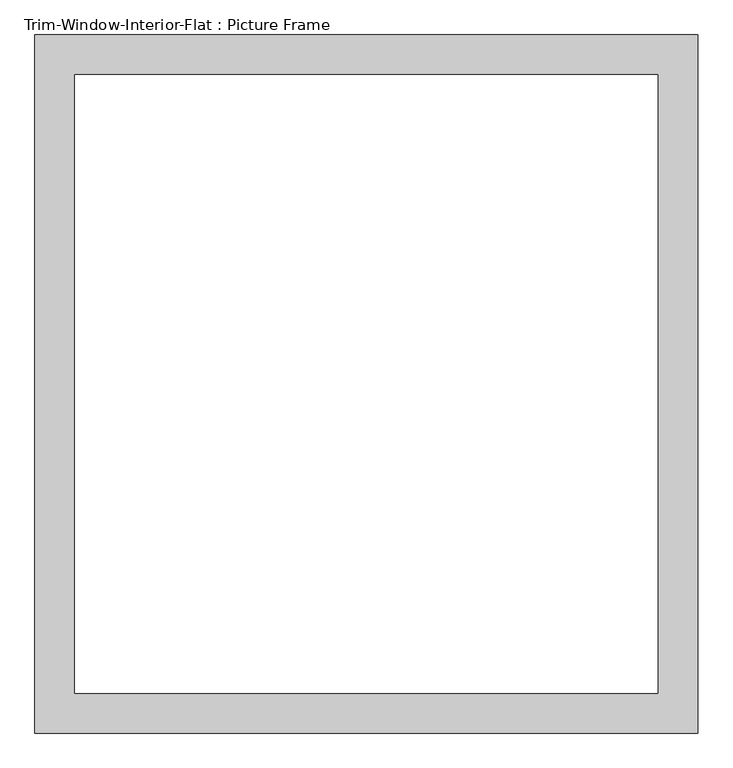
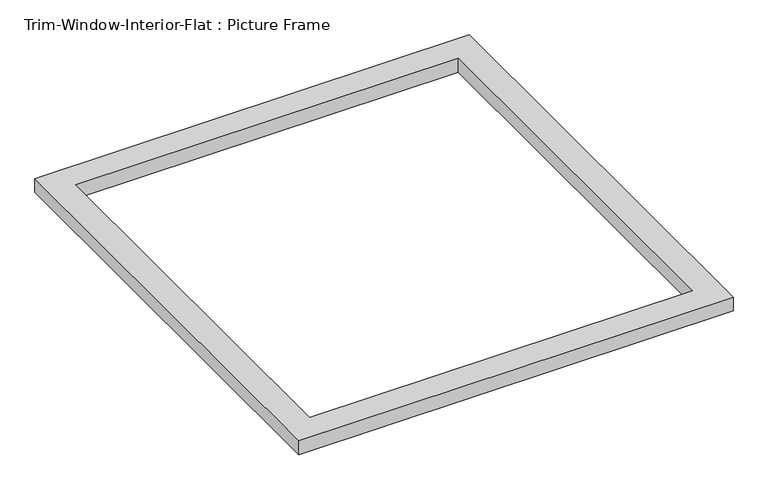
"""IFC4 building model written with IfcOpenShell, lengths in millimetres: proxy geometry, Trim-Window-Interior-Flat : Picture Frame."""

from ifc_helpers import new_model, si_unit, origin, origin_with_axes, place, context, project, spatial, polyline, outline, extrude, source, transform, mapped, element, save


def trim_window_interior_flat_picture_frame_51c85655(model_context):
    return source(origin(), model_context, "Body", "SweptSolid", [
        extrude(outline(polyline([(476.25, 44.45), (476.25, -958.85), (-476.25, -958.85), (-476.25, 44.45), (476.25, 44.45)]), holes=[polyline([(419.1, -12.7), (-419.1, -12.7), (-419.1, -901.7), (419.1, -901.7), (419.1, -12.7)])]), origin_with_axes(), (0.0, 0.0, 1.0), 31.75),
    ])


if __name__ == "__main__":
    model = new_model("IFC4")
    model_context = context("Model", 3, world=origin())
    ifc_project = project(units=[si_unit("LENGTHUNIT", "METRE", prefix="MILLI")], contexts=[model_context])
    site = spatial("IfcSite", under=ifc_project)
    building = spatial("IfcBuilding", under=site)
    placement = place(None, origin())
    trim_window_interior_flat_picture_frame_shape = trim_window_interior_flat_picture_frame_51c85655(model_context)
    element("IfcBuildingElementProxy", 1, Name="Trim-Window-Interior-Flat : Picture Frame", ObjectType="Trim-Window-Interior-Flat : Picture Frame", at=placement, inside=building, context=model_context, shape_type="MappedRepresentation", body=[
        mapped(trim_window_interior_flat_picture_frame_shape, transform((0.0, 0.0, 0.0), x_axis=(1.0, 0.0, 0.0), y_axis=(0.0, 1.0, 0.0), z_axis=(0.0, 0.0, 1.0))),
    ])
    save(model, "model.ifc")

# Revit data of these elements
# Type "Trim-Window-Interior-Flat : Picture Frame"
#   Trim Thickness_Picture Frame = 0' - 1 1/4"
#   Trim Width = 0' - 2 1/4"
#   Trim Thickness_with Sill = 0' - 0 3/4"
#   Sill Thickness = 0' - 1 1/4"
#   Opening Width [instance default] = 2' - 0"
#   Opening Height [instance default] = 3' - 0"
#   Default Elevation = 4' - 0"
#   Sill = no
#   Picture Frame = yes
#   Trim Material [instance default] = none
# Element 1 (IfcBuildingElementProxy, "Trim-Window-Interior-Flat : Picture Frame")
#   Opening Width = 2' - 10"
#   Trim Material = Wood - Stained
#   Materials on its faces: "Wood - Stained"
# Materials
#   "Wood - Stained": class "Wood", colour RGB 224 178 126, transparency 0, Cost = 0
